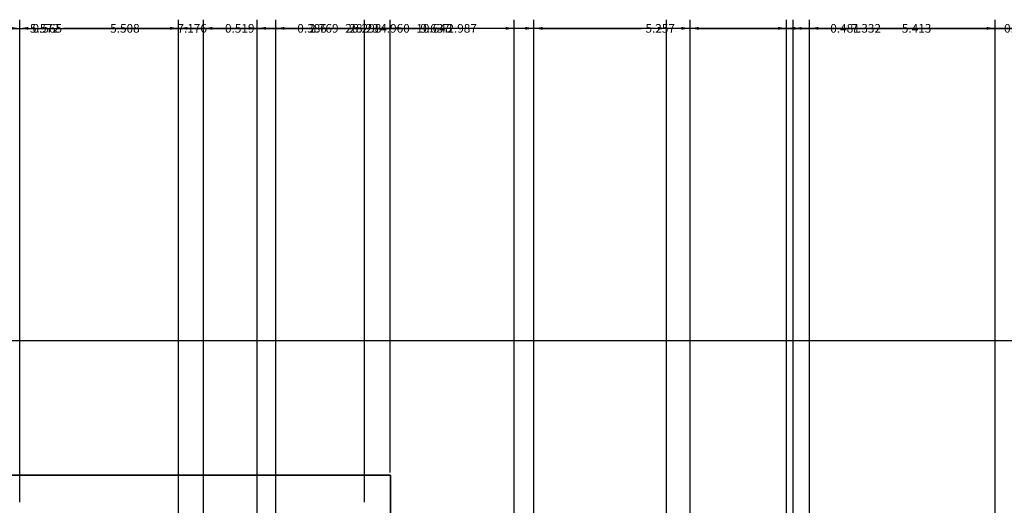
# Model space of a CAD drawing. Units: inches. Extents: x -10 to 130, y -32 to 34.
# Tile 11 of 22: x 29 to 49, y 24 to 34. Entities that reach past the tile are written whole.
import ezdxf

# ---------------------------------------------------------------- set-up
doc = ezdxf.new("R2010")
doc.units = ezdxf.units.IN
doc.header["$MEASUREMENT"] = 0
doc.layers.add('A-ANNO-DIMS', color=2, linetype='Continuous', lineweight=18)
doc.layers.add('A-ELEV', color=7, linetype='Continuous', lineweight=35)
doc.styles.get("Standard").update_dxf_attribs({"font": 'arial.ttf'})
doc.dimstyles.get("Standard").update_dxf_attribs({"dimtxt": 0.18, "dimasz": 0.18, "dimexe": 0.18, "dimexo": 0.0625, "dimgap": 0.09, "dimtad": 0, "dimtih": 1, "dimtoh": 1, "dimdec": 4, "dimzin": 0, "dimdsep": 46, "dimtxsty": 'Standard', "dimcen": 0.09, "dimadec": 0, "dimazin": 0, "dimtfac": 1, "dimtdec": 4, "dimtofl": 0, "dimtmove": 0, "dimatfit": 3, "dimfxl": 1, "dimtolj": 1, "dimtzin": 0, "dimarcsym": 0})

# ---------------------------------------------------------------- blocks, each defined once
blk = doc.blocks.new('*D5')
at = {"layer": 'A-ANNO-DIMS', "color": 0, "lineweight": -2, "transparency": 16777216}
for p, q in [((26.399, 6.07), (26.399, 33.879)), ((31.971, 6.07), (31.971, 33.879)), ((26.579, 33.699), (28.792, 33.699)), ((31.791, 33.699), (29.578, 33.699))]:
    blk.add_line(p, q, dxfattribs=at)
at = {"layer": 'A-ANNO-DIMS', "color": 0, "transparency": 16777216}
for points in [[(26.579, 33.729), (26.579, 33.669), (26.399, 33.699)], [(31.791, 33.729), (31.791, 33.669), (31.971, 33.699)]]:
    blk.add_solid(points, dxfattribs=at)
at = {"layer": 'Defpoints', "color": 0, "transparency": 16777216}
for p in [(31.971, 33.699), (26.399, 6.007), (31.971, 6.007)]:
    blk.add_point(p, dxfattribs=at)
at = {"layer": 'A-ANNO-DIMS', "color": 0, "transparency": 16777216, "insert": (29.185, 33.699), "char_height": 0.18, "attachment_point": 5}
blk.add_mtext('\\A1;5.572', dxfattribs=at)
blk = doc.blocks.new('*D6')
at = {"layer": 'A-ANNO-DIMS', "color": 0, "lineweight": -2, "transparency": 16777216}
for p, q in [((31.971, 6.07), (31.971, 33.879)), ((42.614, 6.07), (42.614, 33.879)), ((32.151, 33.699), (36.837, 33.699)), ((42.434, 33.699), (37.748, 33.699))]:
    blk.add_line(p, q, dxfattribs=at)
at = {"layer": 'A-ANNO-DIMS', "color": 0, "transparency": 16777216}
for points in [[(32.151, 33.729), (32.151, 33.669), (31.971, 33.699)], [(42.434, 33.729), (42.434, 33.669), (42.614, 33.699)]]:
    blk.add_solid(points, dxfattribs=at)
at = {"layer": 'Defpoints', "color": 0, "transparency": 16777216}
for p in [(42.614, 33.699), (31.971, 6.007), (42.614, 6.007)]:
    blk.add_point(p, dxfattribs=at)
at = {"layer": 'A-ANNO-DIMS', "color": 0, "transparency": 16777216, "insert": (37.293, 33.699), "char_height": 0.18, "attachment_point": 5}
blk.add_mtext('\\A1;10.643', dxfattribs=at)
blk = doc.blocks.new('*D7')
at = {"layer": 'A-ANNO-DIMS', "color": 0, "lineweight": -2, "transparency": 16777216}
for p, q in [((42.614, 6.07), (42.614, 33.879)), ((49.946, 6.07), (49.946, 33.879)), ((42.794, 33.699), (45.888, 33.699)), ((49.766, 33.699), (46.672, 33.699))]:
    blk.add_line(p, q, dxfattribs=at)
at = {"layer": 'A-ANNO-DIMS', "color": 0, "transparency": 16777216}
for points in [[(42.794, 33.729), (42.794, 33.669), (42.614, 33.699)], [(49.766, 33.729), (49.766, 33.669), (49.946, 33.699)]]:
    blk.add_solid(points, dxfattribs=at)
at = {"layer": 'Defpoints', "color": 0, "transparency": 16777216}
for p in [(49.946, 33.699), (42.614, 6.007), (49.946, 6.007)]:
    blk.add_point(p, dxfattribs=at)
at = {"layer": 'A-ANNO-DIMS', "color": 0, "transparency": 16777216, "insert": (46.28, 33.699), "char_height": 0.18, "attachment_point": 5}
blk.add_mtext('\\A1;7.332', dxfattribs=at)
blk = doc.blocks.new('*D14')
at = {"layer": 'A-ANNO-DIMS', "color": 0, "lineweight": -2, "transparency": 16777216}
for p, q in [((28.1, 24.464), (28.1, 33.879)), ((33.608, 19.52), (33.608, 33.879)), ((28.28, 33.699), (30.46, 33.699)), ((33.428, 33.699), (31.248, 33.699))]:
    blk.add_line(p, q, dxfattribs=at)
at = {"layer": 'A-ANNO-DIMS', "color": 0, "transparency": 16777216}
for points in [[(28.28, 33.729), (28.28, 33.669), (28.1, 33.699)], [(33.428, 33.729), (33.428, 33.669), (33.608, 33.699)]]:
    blk.add_solid(points, dxfattribs=at)
at = {"layer": 'Defpoints', "color": 0, "transparency": 16777216}
for p in [(33.608, 33.699), (28.1, 24.402), (33.608, 19.458)]:
    blk.add_point(p, dxfattribs=at)
at = {"layer": 'A-ANNO-DIMS', "color": 0, "transparency": 16777216, "insert": (30.854, 33.699), "char_height": 0.18, "attachment_point": 5}
blk.add_mtext('\\A1;5.508', dxfattribs=at)
blk = doc.blocks.new('*D15')
at = {"layer": 'A-ANNO-DIMS', "color": 0, "lineweight": -2, "transparency": 16777216}
for p, q in [((33.608, 19.52), (33.608, 33.879)), ((36.377, 24.464), (36.377, 33.879)), ((33.788, 33.699), (34.597, 33.699)), ((36.197, 33.699), (35.388, 33.699))]:
    blk.add_line(p, q, dxfattribs=at)
at = {"layer": 'A-ANNO-DIMS', "color": 0, "transparency": 16777216}
for points in [[(33.788, 33.729), (33.788, 33.669), (33.608, 33.699)], [(36.197, 33.729), (36.197, 33.669), (36.377, 33.699)]]:
    blk.add_solid(points, dxfattribs=at)
at = {"layer": 'Defpoints', "color": 0, "transparency": 16777216}
for p in [(36.377, 33.699), (36.377, 24.402), (33.608, 19.458)]:
    blk.add_point(p, dxfattribs=at)
at = {"layer": 'A-ANNO-DIMS', "color": 0, "transparency": 16777216, "insert": (34.993, 33.699), "char_height": 0.18, "attachment_point": 5}
blk.add_mtext('\\A1;2.769', dxfattribs=at)
blk = doc.blocks.new('*D16')
at = {"layer": 'A-ANNO-DIMS', "color": 0, "lineweight": -2, "transparency": 16777216}
for p, q in [((36.377, 24.464), (36.377, 33.879)), ((39.364, 19.52), (39.364, 33.879)), ((36.557, 33.699), (37.476, 33.699)), ((39.184, 33.699), (38.266, 33.699))]:
    blk.add_line(p, q, dxfattribs=at)
at = {"layer": 'A-ANNO-DIMS', "color": 0, "transparency": 16777216}
for points in [[(36.557, 33.729), (36.557, 33.669), (36.377, 33.699)], [(39.184, 33.729), (39.184, 33.669), (39.364, 33.699)]]:
    blk.add_solid(points, dxfattribs=at)
at = {"layer": 'Defpoints', "color": 0, "transparency": 16777216}
for p in [(39.364, 33.699), (36.377, 24.402), (39.364, 19.458)]:
    blk.add_point(p, dxfattribs=at)
at = {"layer": 'A-ANNO-DIMS', "color": 0, "transparency": 16777216, "insert": (37.871, 33.699), "char_height": 0.18, "attachment_point": 5}
blk.add_mtext('\\A1;2.987', dxfattribs=at)
blk = doc.blocks.new('*D17')
at = {"layer": 'A-ANNO-DIMS', "color": 0, "lineweight": -2, "transparency": 16777216}
for p, q in [((39.364, 19.52), (39.364, 33.879)), ((44.622, 17.67), (44.622, 33.879)), ((39.544, 33.699), (41.599, 33.699)), ((44.442, 33.699), (42.387, 33.699))]:
    blk.add_line(p, q, dxfattribs=at)
at = {"layer": 'A-ANNO-DIMS', "color": 0, "transparency": 16777216}
for points in [[(39.544, 33.729), (39.544, 33.669), (39.364, 33.699)], [(44.442, 33.729), (44.442, 33.669), (44.622, 33.699)]]:
    blk.add_solid(points, dxfattribs=at)
at = {"layer": 'Defpoints', "color": 0, "transparency": 16777216}
for p in [(44.622, 33.699), (39.364, 19.458), (44.622, 17.607)]:
    blk.add_point(p, dxfattribs=at)
at = {"layer": 'A-ANNO-DIMS', "color": 0, "transparency": 16777216, "insert": (41.993, 33.699), "char_height": 0.18, "attachment_point": 5}
blk.add_mtext('\\A1;5.257', dxfattribs=at)
blk = doc.blocks.new('*D18')
at = {"layer": 'A-ANNO-DIMS', "color": 0, "lineweight": -2, "transparency": 16777216}
for p, q in [((44.622, 17.67), (44.622, 33.879)), ((50.035, 27.261), (50.035, 33.879)), ((44.802, 33.699), (46.935, 33.699)), ((49.855, 33.699), (47.722, 33.699))]:
    blk.add_line(p, q, dxfattribs=at)
at = {"layer": 'A-ANNO-DIMS', "color": 0, "transparency": 16777216}
for points in [[(44.802, 33.729), (44.802, 33.669), (44.622, 33.699)], [(49.855, 33.729), (49.855, 33.669), (50.035, 33.699)]]:
    blk.add_solid(points, dxfattribs=at)
at = {"layer": 'Defpoints', "color": 0, "transparency": 16777216}
for p in [(50.035, 33.699), (50.035, 27.199), (44.622, 17.607)]:
    blk.add_point(p, dxfattribs=at)
at = {"layer": 'A-ANNO-DIMS', "color": 0, "transparency": 16777216, "insert": (47.328, 33.699), "char_height": 0.18, "attachment_point": 5}
blk.add_mtext('\\A1;5.413', dxfattribs=at)
blk = doc.blocks.new('*D28')
at = {"layer": 'A-ANNO-DIMS', "color": 0, "lineweight": -2, "transparency": 16777216}
for p, q in [((21.715, 14.903), (21.715, 33.879)), ((49.946, 14.903), (49.946, 33.879)), ((21.895, 33.699), (35.436, 33.699)), ((49.766, 33.699), (36.226, 33.699))]:
    blk.add_line(p, q, dxfattribs=at)
at = {"layer": 'A-ANNO-DIMS', "color": 0, "transparency": 16777216}
for points in [[(21.895, 33.729), (21.895, 33.669), (21.715, 33.699)], [(49.766, 33.729), (49.766, 33.669), (49.946, 33.699)]]:
    blk.add_solid(points, dxfattribs=at)
at = {"layer": 'Defpoints', "color": 0, "transparency": 16777216}
for p in [(49.946, 33.699), (21.715, 14.841), (49.946, 14.841)]:
    blk.add_point(p, dxfattribs=at)
at = {"layer": 'A-ANNO-DIMS', "color": 0, "transparency": 16777216, "insert": (35.831, 33.699), "char_height": 0.18, "attachment_point": 5}
blk.add_mtext('\\A1;28.23', dxfattribs=at)
blk = doc.blocks.new('*D39')
at = {"layer": 'A-ANNO-DIMS', "color": 0, "lineweight": -2, "transparency": 16777216}
for p, q in [((49.972, 27.199), (-9.564, 27.199)), ((-9.384, 27.019), (-9.384, 25.982)), ((-9.384, 24.582), (-9.384, 25.618)), ((28.037, 24.402), (-9.564, 24.402))]:
    blk.add_line(p, q, dxfattribs=at)
at = {"layer": 'A-ANNO-DIMS', "color": 0, "transparency": 16777216}
for points in [[(-9.414, 27.019), (-9.354, 27.019), (-9.384, 27.199)], [(-9.414, 24.582), (-9.354, 24.582), (-9.384, 24.402)]]:
    blk.add_solid(points, dxfattribs=at)
at = {"layer": 'Defpoints', "color": 0, "transparency": 16777216}
for p in [(-9.384, 27.199), (50.035, 27.199), (28.1, 24.402)]:
    blk.add_point(p, dxfattribs=at)
at = {"layer": 'A-ANNO-DIMS', "color": 0, "transparency": 16777216, "insert": (-9.384, 25.8), "char_height": 0.18, "attachment_point": 5}
blk.add_mtext('\\A1;2.797', dxfattribs=at)
blk = doc.blocks.new('*D48')
at = {"layer": 'A-ANNO-DIMS', "color": 0, "lineweight": -2, "transparency": 16777216}
for p, q in [((44.76, -13.293), (44.76, 33.879)), ((74.492, -13.293), (74.492, 33.879)), ((44.94, 33.699), (59.231, 33.699)), ((74.312, 33.699), (60.021, 33.699))]:
    blk.add_line(p, q, dxfattribs=at)
at = {"layer": 'A-ANNO-DIMS', "color": 0, "transparency": 16777216}
for points in [[(44.94, 33.729), (44.94, 33.669), (44.76, 33.699)], [(74.312, 33.729), (74.312, 33.669), (74.492, 33.699)]]:
    blk.add_solid(points, dxfattribs=at)
at = {"layer": 'Defpoints', "color": 0, "transparency": 16777216}
for p in [(74.492, 33.699), (44.76, -13.356), (74.492, -13.356)]:
    blk.add_point(p, dxfattribs=at)
at = {"layer": 'A-ANNO-DIMS', "color": 0, "transparency": 16777216, "insert": (59.626, 33.699), "char_height": 0.18, "attachment_point": 5}
blk.add_mtext('\\A1;29.73', dxfattribs=at)
blk = doc.blocks.new('*D99')
at = {"layer": 'A-ANNO-DIMS', "color": 0, "lineweight": -2, "transparency": 16777216}
for p, q in [((28.1, 24.464), (28.1, 33.879)), ((28.665, 23.841), (28.665, 33.879)), ((28.28, 33.699), (28.485, 33.699)), ((28.665, 33.699), (28.845, 33.699))]:
    blk.add_line(p, q, dxfattribs=at)
at = {"layer": 'A-ANNO-DIMS', "color": 0, "transparency": 16777216}
for points in [[(28.28, 33.729), (28.28, 33.669), (28.1, 33.699)], [(28.485, 33.729), (28.485, 33.669), (28.665, 33.699)]]:
    blk.add_solid(points, dxfattribs=at)
at = {"layer": 'Defpoints', "color": 0, "transparency": 16777216}
for p in [(28.665, 33.699), (28.1, 24.402), (28.665, 23.779)]:
    blk.add_point(p, dxfattribs=at)
at = {"layer": 'A-ANNO-DIMS', "color": 0, "transparency": 16777216, "insert": (29.239, 33.699), "char_height": 0.18, "attachment_point": 5}
blk.add_mtext('\\A1;0.565', dxfattribs=at)
blk = doc.blocks.new('*D100')
at = {"layer": 'A-ANNO-DIMS', "color": 0, "lineweight": -2, "transparency": 16777216}
for p, q in [((28.665, 23.841), (28.665, 33.879)), ((35.841, 23.841), (35.841, 33.879)), ((28.845, 33.699), (31.86, 33.699)), ((35.661, 33.699), (32.646, 33.699))]:
    blk.add_line(p, q, dxfattribs=at)
at = {"layer": 'A-ANNO-DIMS', "color": 0, "transparency": 16777216}
for points in [[(28.845, 33.729), (28.845, 33.669), (28.665, 33.699)], [(35.661, 33.729), (35.661, 33.669), (35.841, 33.699)]]:
    blk.add_solid(points, dxfattribs=at)
at = {"layer": 'Defpoints', "color": 0, "transparency": 16777216}
for p in [(35.841, 33.699), (28.665, 23.779), (35.841, 23.779)]:
    blk.add_point(p, dxfattribs=at)
at = {"layer": 'A-ANNO-DIMS', "color": 0, "transparency": 16777216, "insert": (32.253, 33.699), "char_height": 0.18, "attachment_point": 5}
blk.add_mtext('\\A1;7.176', dxfattribs=at)
blk = doc.blocks.new('*D102')
at = {"layer": 'A-ANNO-DIMS', "color": 0, "lineweight": -2, "transparency": 16777216}
for p, q in [((33.608, 19.52), (33.608, 33.879)), ((33.994, 18.998), (33.994, 33.879)), ((33.428, 33.699), (33.248, 33.699)), ((34.174, 33.699), (34.354, 33.699))]:
    blk.add_line(p, q, dxfattribs=at)
at = {"layer": 'A-ANNO-DIMS', "color": 0, "transparency": 16777216}
for points in [[(33.428, 33.729), (33.428, 33.669), (33.608, 33.699)], [(34.174, 33.729), (34.174, 33.669), (33.994, 33.699)]]:
    blk.add_solid(points, dxfattribs=at)
at = {"layer": 'Defpoints', "color": 0, "transparency": 16777216}
for p in [(33.994, 33.699), (33.608, 19.458), (33.994, 18.936)]:
    blk.add_point(p, dxfattribs=at)
at = {"layer": 'A-ANNO-DIMS', "color": 0, "transparency": 16777216, "insert": (34.748, 33.699), "char_height": 0.18, "attachment_point": 5}
blk.add_mtext('\\A1;0.386', dxfattribs=at)
blk = doc.blocks.new('*D103')
at = {"layer": 'A-ANNO-DIMS', "color": 0, "lineweight": -2, "transparency": 16777216}
for p, q in [((33.994, 18.998), (33.994, 33.879)), ((38.954, 18.998), (38.954, 33.879)), ((34.174, 33.699), (36.077, 33.699)), ((38.774, 33.699), (36.871, 33.699))]:
    blk.add_line(p, q, dxfattribs=at)
at = {"layer": 'A-ANNO-DIMS', "color": 0, "transparency": 16777216}
for points in [[(34.174, 33.729), (34.174, 33.669), (33.994, 33.699)], [(38.774, 33.729), (38.774, 33.669), (38.954, 33.699)]]:
    blk.add_solid(points, dxfattribs=at)
at = {"layer": 'Defpoints', "color": 0, "transparency": 16777216}
for p in [(38.954, 33.699), (33.994, 18.936), (38.954, 18.936)]:
    blk.add_point(p, dxfattribs=at)
at = {"layer": 'A-ANNO-DIMS', "color": 0, "transparency": 16777216, "insert": (36.474, 33.699), "char_height": 0.18, "attachment_point": 5}
blk.add_mtext('\\A1;4.960', dxfattribs=at)
blk = doc.blocks.new('*D106')
at = {"layer": 'A-ANNO-DIMS', "color": 0, "lineweight": -2, "transparency": 16777216}
for p, q in [((22.665, 14.318), (22.665, 33.879)), ((48.963, 14.318), (48.963, 33.879)), ((22.845, 33.699), (35.349, 33.699)), ((48.783, 33.699), (36.279, 33.699))]:
    blk.add_line(p, q, dxfattribs=at)
at = {"layer": 'A-ANNO-DIMS', "color": 0, "transparency": 16777216}
for points in [[(22.845, 33.729), (22.845, 33.669), (22.665, 33.699)], [(48.783, 33.729), (48.783, 33.669), (48.963, 33.699)]]:
    blk.add_solid(points, dxfattribs=at)
at = {"layer": 'Defpoints', "color": 0, "transparency": 16777216}
for p in [(48.963, 33.699), (22.665, 14.256), (48.963, 14.256)]:
    blk.add_point(p, dxfattribs=at)
at = {"layer": 'A-ANNO-DIMS', "color": 0, "transparency": 16777216, "insert": (35.814, 33.699), "char_height": 0.18, "attachment_point": 5}
blk.add_mtext('\\A1;26.298', dxfattribs=at)
blk = doc.blocks.new('*D107')
at = {"layer": 'A-ANNO-DIMS', "color": 0, "lineweight": -2, "transparency": 16777216}
for p, q in [((48.963, 14.318), (48.963, 33.879)), ((49.946, 14.903), (49.946, 33.879)), ((48.783, 33.699), (48.603, 33.699)), ((50.126, 33.699), (50.306, 33.699))]:
    blk.add_line(p, q, dxfattribs=at)
at = {"layer": 'A-ANNO-DIMS', "color": 0, "transparency": 16777216}
for points in [[(48.783, 33.729), (48.783, 33.669), (48.963, 33.699)], [(50.126, 33.729), (50.126, 33.669), (49.946, 33.699)]]:
    blk.add_solid(points, dxfattribs=at)
at = {"layer": 'Defpoints', "color": 0, "transparency": 16777216}
for p in [(49.946, 33.699), (49.946, 14.841), (48.963, 14.256)]:
    blk.add_point(p, dxfattribs=at)
at = {"layer": 'A-ANNO-DIMS', "color": 0, "transparency": 16777216, "insert": (49.455, 33.699), "char_height": 0.18, "attachment_point": 5}
blk.add_mtext('\\A1;0.983', dxfattribs=at)
blk = doc.blocks.new('*D109')
at = {"layer": 'A-ANNO-DIMS', "color": 0, "lineweight": -2, "transparency": 16777216}
for p, q in [((44.622, 17.67), (44.622, 33.879)), ((45.103, 17.205), (45.103, 33.879)), ((44.442, 33.699), (44.262, 33.699)), ((45.283, 33.699), (45.463, 33.699))]:
    blk.add_line(p, q, dxfattribs=at)
at = {"layer": 'A-ANNO-DIMS', "color": 0, "transparency": 16777216}
for points in [[(44.442, 33.729), (44.442, 33.669), (44.622, 33.699)], [(45.283, 33.729), (45.283, 33.669), (45.103, 33.699)]]:
    blk.add_solid(points, dxfattribs=at)
at = {"layer": 'Defpoints', "color": 0, "transparency": 16777216}
for p in [(45.103, 33.699), (44.622, 17.607), (45.103, 17.143)]:
    blk.add_point(p, dxfattribs=at)
at = {"layer": 'A-ANNO-DIMS', "color": 0, "transparency": 16777216, "insert": (45.839, 33.699), "char_height": 0.18, "attachment_point": 5}
blk.add_mtext('\\A1;0.481', dxfattribs=at)
blk = doc.blocks.new('*D119')
at = {"layer": 'A-ANNO-DIMS', "color": 0, "lineweight": -2, "transparency": 16777216}
for p, q in [((31.971, 6.07), (31.971, 33.879)), ((32.49, 5.634), (32.49, 33.879)), ((31.791, 33.699), (31.611, 33.699)), ((32.67, 33.699), (32.85, 33.699))]:
    blk.add_line(p, q, dxfattribs=at)
at = {"layer": 'A-ANNO-DIMS', "color": 0, "transparency": 16777216}
for points in [[(31.791, 33.729), (31.791, 33.669), (31.971, 33.699)], [(32.67, 33.729), (32.67, 33.669), (32.49, 33.699)]]:
    blk.add_solid(points, dxfattribs=at)
at = {"layer": 'Defpoints', "color": 0, "transparency": 16777216}
for p in [(32.49, 33.699), (31.971, 6.007), (32.49, 5.572)]:
    blk.add_point(p, dxfattribs=at)
at = {"layer": 'A-ANNO-DIMS', "color": 0, "transparency": 16777216, "insert": (33.244, 33.699), "char_height": 0.18, "attachment_point": 5}
blk.add_mtext('\\A1;0.519', dxfattribs=at)
blk = doc.blocks.new('*D120')
at = {"layer": 'A-ANNO-DIMS', "color": 0, "lineweight": -2, "transparency": 16777216}
for p, q in [((32.49, 5.634), (32.49, 33.879)), ((42.127, 5.634), (42.127, 33.879)), ((32.67, 33.699), (36.915, 33.699)), ((41.947, 33.699), (37.702, 33.699))]:
    blk.add_line(p, q, dxfattribs=at)
at = {"layer": 'A-ANNO-DIMS', "color": 0, "transparency": 16777216}
for points in [[(32.67, 33.729), (32.67, 33.669), (32.49, 33.699)], [(41.947, 33.729), (41.947, 33.669), (42.127, 33.699)]]:
    blk.add_solid(points, dxfattribs=at)
at = {"layer": 'Defpoints', "color": 0, "transparency": 16777216}
for p in [(42.127, 33.699), (32.49, 5.572), (42.127, 5.572)]:
    blk.add_point(p, dxfattribs=at)
at = {"layer": 'A-ANNO-DIMS', "color": 0, "transparency": 16777216, "insert": (37.308, 33.699), "char_height": 0.18, "attachment_point": 5}
blk.add_mtext('\\A1;9.637', dxfattribs=at)

msp = doc.modelspace()

# ---------------------------------------------------------------- linework, layer by layer
at = {"layer": 'A-ELEV'}
for p, q in [((28.0997, 24.4019), (36.3774, 24.4019)), ((36.3774, 24.4019), (36.3774, 19.4575))]:
    msp.add_line(p, q, dxfattribs=at)

# ---------------------------------------------------------------- dimensions: what is measured, and where the dimension line sits
at = {"layer": 'A-ANNO-DIMS'}
for base, p1, p2, override, picture, middle in [((49.9462, 33.6987), (21.7155, 14.8409), (49.9462, 14.8409), {"dimdec": 2, "dimlfac": 1, "dimrnd": 0, "dimzin": 0, "dimdsep": 46, "dimlunit": 2}, '*D28', (35.8308, 33.6987)), ((48.963, 33.6987), (22.6649, 14.2556), (48.963, 14.2556), {"dimdec": 3, "dimlfac": 1, "dimrnd": 0, "dimzin": 0, "dimdsep": 46, "dimlunit": 2}, '*D106', (35.8139, 33.6987)), ((31.9712, 33.6987), (26.3988, 6.0074), (31.9712, 6.0074), {"dimdec": 3, "dimlfac": 1, "dimrnd": 0, "dimzin": 0, "dimdsep": 46, "dimlunit": 2}, '*D5', (29.185, 33.6987)), ((33.60816, 33.69866), (28.0997, 24.40191), (33.60816, 19.45752), {"dimdec": 3, "dimlfac": 1, "dimrnd": 0, "dimzin": 0, "dimdsep": 46, "dimlunit": 2}, '*D14', (30.85393, 33.69866)), ((28.6645, 33.6987), (28.0997, 24.4019), (28.6645, 23.7785), {"dimdec": 3, "dimlfac": 1, "dimrnd": 0, "dimzin": 0, "dimdsep": 46, "dimlunit": 2}, '*D99', (29.2389, 33.6987)), ((35.84098, 33.69866), (28.66453, 23.77854), (35.84098, 23.77854), {"dimdec": 3, "dimlfac": 1, "dimrnd": 0, "dimzin": 0, "dimdsep": 46, "dimlunit": 2}, '*D100', (32.25276, 33.69866)), ((32.4898, 33.6987), (31.9712, 6.0074), (32.4898, 5.5715), {"dimdec": 3, "dimlfac": 1, "dimrnd": 0, "dimzin": 0, "dimdsep": 46, "dimlunit": 2}, '*D119', (33.2437, 33.6987)), ((42.614, 33.6987), (31.9712, 6.0074), (42.614, 6.0074), {"dimdec": 3, "dimlfac": 1, "dimrnd": 0, "dimzin": 0, "dimdsep": 46, "dimlunit": 2}, '*D6', (37.2926, 33.6987)), ((42.1266, 33.6987), (32.4898, 5.5715), (42.1266, 5.5715), {"dimdec": 3, "dimlfac": 1, "dimrnd": 0, "dimzin": 0, "dimdsep": 46, "dimlunit": 2}, '*D120', (37.3082, 33.6987)), ((33.994, 33.6987), (33.6082, 19.4575), (33.994, 18.9359), {"dimdec": 3, "dimlfac": 1, "dimrnd": 0, "dimzin": 0, "dimdsep": 46, "dimlunit": 2}, '*D102', (34.7476, 33.6987)), ((36.3774, 33.6987), (33.6082, 19.4575), (36.3774, 24.4019), {"dimdec": 3, "dimlfac": 1, "dimrnd": 0, "dimzin": 0, "dimdsep": 46, "dimlunit": 2}, '*D15', (34.9928, 33.6987)), ((38.95445, 33.69866), (33.99396, 18.93588), (38.95445, 18.93588), {"dimdec": 3, "dimlfac": 1, "dimrnd": 0, "dimzin": 0, "dimdsep": 46, "dimlunit": 2}, '*D103', (36.4742, 33.69866)), ((39.3644, 33.6987), (36.3774, 24.4019), (39.3644, 19.4575), {"dimdec": 3, "dimlfac": 1, "dimrnd": 0, "dimzin": 0, "dimdsep": 46, "dimlunit": 2}, '*D16', (37.8709, 33.6987)), ((44.6217, 33.6987), (39.3644, 19.4575), (44.6217, 17.6074), {"dimdec": 3, "dimlfac": 1, "dimrnd": 0, "dimzin": 0, "dimdsep": 46, "dimlunit": 2}, '*D17', (41.9931, 33.6987)), ((49.9462, 33.6987), (42.614, 6.0074), (49.9462, 6.0074), {"dimdec": 3, "dimlfac": 1, "dimrnd": 0, "dimzin": 0, "dimdsep": 46, "dimlunit": 2}, '*D7', (46.2801, 33.6987)), ((45.1026, 33.6987), (44.6217, 17.6074), (45.1026, 17.1427), {"dimdec": 3, "dimlfac": 1, "dimrnd": 0, "dimzin": 0, "dimdsep": 46, "dimlunit": 2}, '*D109', (45.8389, 33.6987)), ((50.0347, 33.6987), (44.6217, 17.6074), (50.0347, 27.1987), {"dimdec": 3, "dimlfac": 1, "dimrnd": 0, "dimzin": 0, "dimdsep": 46, "dimlunit": 2}, '*D18', (47.3282, 33.6987)), ((74.492, 33.6987), (44.76, -13.3558), (74.492, -13.3558), {"dimdec": 2, "dimlfac": 1, "dimrnd": 0, "dimzin": 0, "dimdsep": 46, "dimlunit": 2}, '*D48', (59.626, 33.6987)), ((49.9462, 33.6987), (48.963, 14.2556), (49.9462, 14.8409), {"dimdec": 3, "dimlfac": 1, "dimrnd": 0, "dimzin": 0, "dimdsep": 46, "dimlunit": 2}, '*D107', (49.4546, 33.6987))]:
    dim = msp.add_linear_dim(base=base, p1=p1, p2=p2, dimstyle='Standard', override=override, dxfattribs=at)
    dim.commit()
    dim.dimension.update_dxf_attribs({"geometry": picture, "text_midpoint": middle})
dim = msp.add_linear_dim(base=(-9.3836, 27.1987), p1=(28.0997, 24.4019), p2=(50.0347, 27.1987), angle=90, dimstyle='Standard', override={"dimdec": 3, "dimlfac": 1, "dimrnd": 0, "dimzin": 0, "dimdsep": 46, "dimlunit": 2}, dxfattribs=at)
dim.commit()
dim.dimension.update_dxf_attribs({"geometry": '*D39', "text_midpoint": (-9.3836, 25.8003)})

doc.saveas('drawing.dxf')
